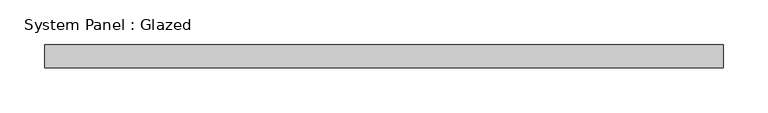
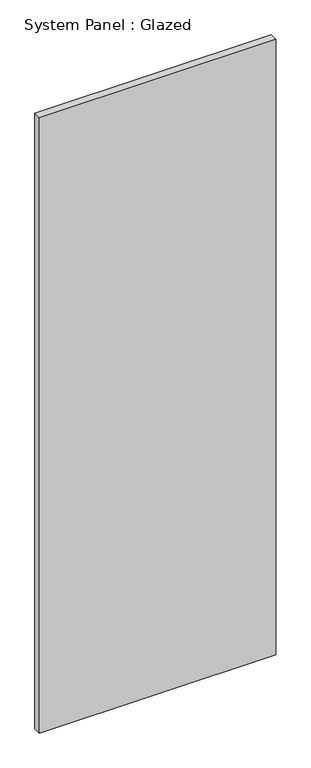
"""IFC4 building model written with IfcOpenShell, lengths in millimetres: plate geometry, System Panel : Glazed."""

from ifc_helpers import new_model, si_unit, origin, origin_with_axes, place, context, project, spatial, polyline, outline, extrude, source, transform, mapped, element, save


def system_panel_glazed_3c43e7a7(model_context):
    return source(origin(), model_context, "Body", "SweptSolid", [
        extrude(outline(polyline([(377.825, 19.05), (-377.825, 19.05), (-377.825, 44.45), (377.825, 44.45), (377.825, 19.05)])), origin_with_axes(), (0.0, 0.0, 1.0), 2081.0093941),
    ])


if __name__ == "__main__":
    model = new_model("IFC4")
    model_context = context("Model", 3, world=origin())
    ifc_project = project(units=[si_unit("LENGTHUNIT", "METRE", prefix="MILLI")], contexts=[model_context])
    site = spatial("IfcSite", under=ifc_project)
    building = spatial("IfcBuilding", under=site)
    placement = place(None, origin())
    system_panel_glazed_shape = system_panel_glazed_3c43e7a7(model_context)
    element("IfcPlate", 1, ObjectType="System Panel : Glazed", at=placement, inside=building, context=model_context, shape_type="MappedRepresentation", body=[
        mapped(system_panel_glazed_shape, transform((0.0, 0.0, 0.0), x_axis=(1.0, 0.0, 0.0), y_axis=(0.0, 1.0, 0.0), z_axis=(0.0, 0.0, 1.0))),
    ])
    save(model, "model.ifc")

# Revit data of these elements
# Type "System Panel : Glazed"
#   Construction Type Id = "GSP4R"
#   Analytic Construction = "1/8 in Pilkington single glazing"
#   Visual Light Transmittance = 0.9
#   Solar Heat Gain Coefficient = 0.86
#   Heat Transfer Coefficient (U) = 1.18115 BTU/(h·ft²·°F)
#   Define Thermal Properties by = 1
# Element 1 (IfcPlate, "System Panel : Glazed")
#   Materials on its faces: "Glass"
# Materials
#   "Glass": class "Glass", colour RGB 0 128 192, transparency 0.75, Description = "Soda Lime Glass", Cost = 0
